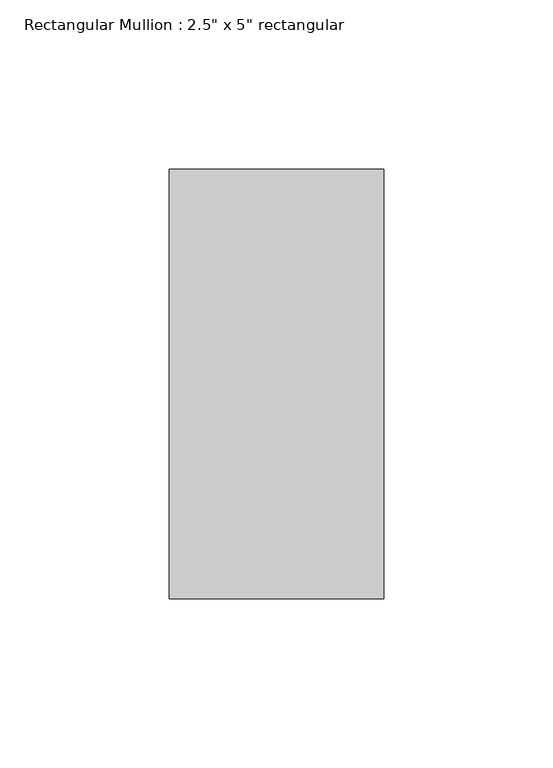
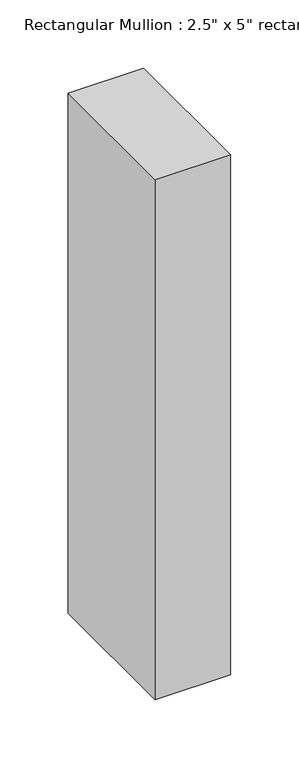
"""IFC4 building model written with IfcOpenShell, lengths in millimetres: member geometry."""

from ifc_helpers import new_model, si_unit, frame, origin, place, context, project, spatial, polyline, outline, extrude, source, transform, mapped, element, save


def member_1df11e17(model_context):
    return source(origin(), model_context, "Body", "SweptSolid", [
        extrude(outline(polyline([(31.75, 63.5), (31.75, -63.5), (-31.75, -63.5), (-31.75, 63.5), (31.75, 63.5)])), frame((0.0, 0.0, -463.55), z_axis=(0.0, 0.0, 1.0), x_axis=(1.0, 0.0, 0.0)), (0.0, 0.0, 1.0), 463.55),
    ])


if __name__ == "__main__":
    model = new_model("IFC4")
    model_context = context("Model", 3, world=origin())
    ifc_project = project(units=[si_unit("LENGTHUNIT", "METRE", prefix="MILLI")], contexts=[model_context])
    site = spatial("IfcSite", under=ifc_project)
    building = spatial("IfcBuilding", under=site)
    placement = place(None, origin())
    member_shape = member_1df11e17(model_context)
    element("IfcMember", 1, ObjectType="Rectangular Mullion : 2.5\" x 5\" rectangular", at=placement, inside=building, context=model_context, shape_type="MappedRepresentation", body=[
        mapped(member_shape, transform((0.0, 0.0, 0.0), x_axis=(1.0, 0.0, 0.0), y_axis=(0.0, 1.0, 0.0), z_axis=(0.0, 0.0, 1.0))),
    ])
    save(model, "model.ifc")

# Revit data of these elements
# Type "Rectangular Mullion : 2.5\" x 5\" rectangular"
#   built-in parameter 1007304 = 0.416667 (stored number, unit not read)
#   built-in parameter 1007301 = 0.104167 (stored number, unit not read)
#   built-in parameter 1007300 = 0.104167 (stored number, unit not read)
# Element 1 (IfcMember, "Rectangular Mullion : 2.5\" x 5\" rectangular")
#   Materials on its faces: "Aluminum"
# Materials
#   "Aluminum": class "Metal", colour RGB 247 247 247, transparency 0, Description = "Aluminum 6061", Cost = 0
